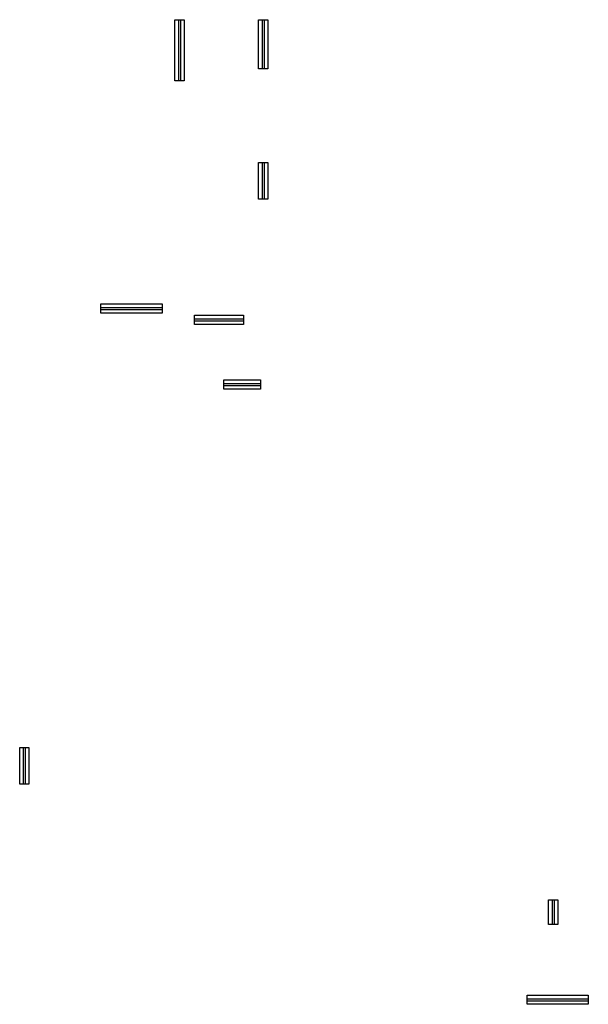
# Model space of a CAD drawing. Units: inches. Extents: x 626 to 5030, y -1681 to 1720.
# Tile 1 of 5: x 626 to 1184, y -1681 to -716. Entities that reach past the tile are written whole.
import ezdxf

# ---------------------------------------------------------------- set-up
doc = ezdxf.new("R2010")
doc.units = ezdxf.units.IN
doc.header["$MEASUREMENT"] = 0
doc.layers.add('A-GLAZ', color=4, linetype='Continuous', lineweight=25)
doc.layers.add('windows', color=4, linetype='Continuous')

# ---------------------------------------------------------------- blocks, each defined once
blk = doc.blocks.new('WINDOW')
at = {"layer": 'windows'}
for p, q in [((173.55, 537.52), (173.55, 489.52)), ((175.55, 537.52), (175.55, 489.52))]:
    blk.add_line(p, q, dxfattribs=at)
blk.add_lwpolyline([(170.05, 537.52), (179.05, 537.52), (179.05, 489.52), (170.05, 489.52)], close=True, dxfattribs=at)
blk = doc.blocks.new('W3')
at = {"layer": 'windows'}
for p, q in [((2120.1, 414.87), (2120.1, 378.87)), ((2122.1, 414.87), (2122.1, 378.87))]:
    blk.add_line(p, q, dxfattribs=at)
blk.add_lwpolyline([(2116.6, 414.87), (2125.6, 414.87), (2125.6, 378.87), (2116.6, 378.87)], close=True, dxfattribs=at)
blk = doc.blocks.new('W5')
at = {"layer": 'windows'}
for p, q in [((2038.16, 554.88), (2038.16, 494.88)), ((2040.16, 554.88), (2040.16, 494.88))]:
    blk.add_line(p, q, dxfattribs=at)
blk.add_lwpolyline([(2034.66, 554.88), (2043.66, 554.88), (2043.66, 494.88), (2034.66, 494.88)], close=True, dxfattribs=at)
blk = doc.blocks.new('V1')
at = {"layer": 'windows'}
for p, q in [((3301.5, 317.53), (3301.5, 293.53)), ((3303.5, 317.53), (3303.5, 293.53))]:
    blk.add_line(p, q, dxfattribs=at)
blk.add_lwpolyline([(3298, 317.53), (3307, 317.53), (3307, 293.53), (3298, 293.53)], close=True, dxfattribs=at)

msp = doc.modelspace()

# ---------------------------------------------------------------- block references
at = {"layer": 'A-GLAZ'}
for name, p in [('W5', (-1255.9, -1271)), ('WINDOW', (690.65, -1253.65)), ('W3', (-1255.9, -1271)), ('W3', (-1490.11, -1844.4)), ('V1', (-2152.9, -1896.5))]:
    msp.add_blockref(name, p, dxfattribs=at)
at = {"layer": 'A-GLAZ', "rotation": 90}
for name, p in [('W5', (1260.97, -3038.45)), ('WINDOW', (1335.29, -1184.81)), ('W3', (1241.41, -3194.85)), ('W5', (1678.89, -3715.89))]:
    msp.add_blockref(name, p, dxfattribs=at)

doc.saveas('drawing.dxf')
